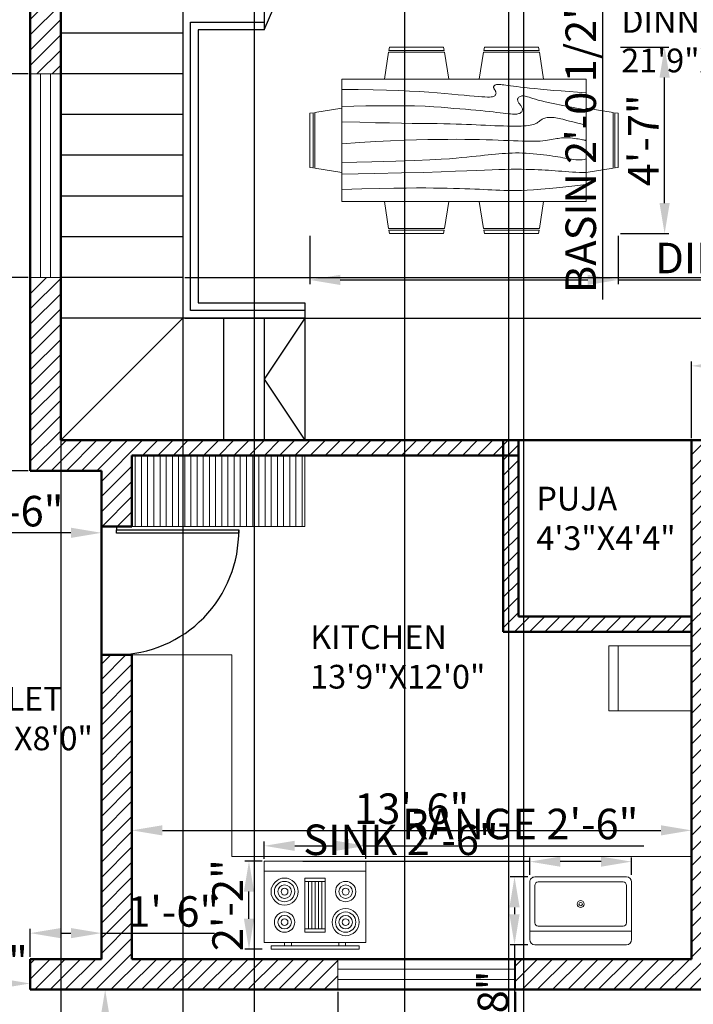
# Model space of a CAD drawing. Units: inches. Extents: x 53662 to 54269, y 37303 to 38048.
# Tile 3 of 6: x 53780 to 53979, y 37459 to 37749. Entities that reach past the tile are written whole.
import ezdxf

# ---------------------------------------------------------------- set-up
doc = ezdxf.new("R2010")
doc.units = ezdxf.units.IN
for name, color, linetype, lineweight in [('A-ANNO-DIMS', 2, 'Continuous', 18), ('A-AREA-IDEN', 7, 'Continuous', 25), ('A-CASE-PATT', 8, 'Continuous', 13), ('A-DOOR', 3, 'Continuous', 25), ('A-EQPM', 9, 'Continuous', 18), ('A-FLOR-CASE', 8, 'Continuous', 18), ('A-FLOR-FIXT', 9, 'Continuous', 18), ('A-FLOR-STRS', 7, 'Continuous', 25), ('A-FURN', 8, 'Continuous', 18), ('A-GLAZ', 4, 'Continuous', 18), ('A-WALL', 7, 'Continuous', 50)]:
    doc.layers.add(name, color=color, linetype=linetype, lineweight=lineweight)
doc.layers.add('A-WALL-PATT', color=244, linetype='Continuous', lineweight=13, true_color=0x991b1e)
doc.styles.get("Standard").update_dxf_attribs({"font": 'arial.ttf'})
doc.dimstyles.new('ISO-25', dxfattribs={"dimtxt": 9, "dimasz": 9, "dimexe": 1.25, "dimexo": 0.625, "dimtad": 1, "dimdec": 1, "dimrnd": 9, "dimlunit": 3, "dimtxsty": 'Standard', "dimcen": 2.5, "dimadec": 0, "dimazin": 0, "dimtfac": 1, "dimtdec": 1, "dimtmove": 0, "dimatfit": 3, "dimfxl": 1, "dimarcsym": 0})

# ---------------------------------------------------------------- blocks, each defined once
blk = doc.blocks.new('Dining Set - 36 x 72 in.')
for p, q in [((-22, 27.5), (-22.1562, 26.50042)), ((-5.8416, 26.5), (-22.1534, 26.5)), ((-22, 27.5), (-6, 27.5)), ((-5.8437, 26.49966), (-6, 27.5)), ((6, 27.5), (5.8438, 26.50042)), ((22.1584, 26.5), (5.8466, 26.5)), ((6, 27.5), (22, 27.5)), ((22.1563, 26.49966), (22, 27.5)), ((-22.2343, 26.00059), (-23.4847, 17.99762)), ((-22.2304, 26), (-5.7608, 26)), ((-4.5152, 17.99762), (-5.7655, 25.99926)), ((5.7657, 26.00059), (4.5153, 17.99762)), ((5.7696, 26), (22.2392, 26)), ((23.4848, 17.99762), (22.2345, 25.99926)), ((36, 18), (-36, 18)), ((-36, 18), (-36, -18)), ((36, -18), (36, 18)), ((-44.0006, 8.23428), (-35.9976, 9.48474)), ((44.0006, 8.23428), (35.9976, 9.48474)), ((-45.5, 8), (-44.5004, 8.15617)), ((-45.5, 8), (-45.5, -8)), ((-44.5, -8.15843), (-44.5, 8.15338)), ((-44, 8.23041), (-44, -8.23915)), ((44, 8.23041), (44, -8.23915)), ((44.5, -8.15843), (44.5, 8.15338)), ((45.5, 8), (44.5005, 8.15617)), ((45.5, 8), (45.5, -8)), ((-44.4997, -8.15631), (-45.5, -8)), ((-35.9976, -9.48476), (-43.9993, -8.2345)), ((35.9976, -9.48476), (43.9993, -8.2345)), ((44.4997, -8.15631), (45.5, -8)), ((-36, -18), (36, -18)), ((-22.2343, -26.0006), (-23.4847, -17.99762)), ((-4.5152, -17.99762), (-5.7655, -25.99928)), ((5.7657, -26.0006), (4.5153, -17.99762)), ((23.4848, -17.99762), (22.2345, -25.99928)), ((-22.2304, -26), (-5.7608, -26)), ((5.7696, -26), (22.2392, -26)), ((-22, -27.5), (-22.1562, -26.50044)), ((-5.8416, -26.5), (-22.1534, -26.5)), ((-22, -27.5), (-6, -27.5)), ((-5.8437, -26.49967), (-6, -27.5)), ((6, -27.5), (5.8438, -26.50044)), ((22.1584, -26.5), (5.8466, -26.5)), ((6, -27.5), (22, -27.5)), ((22.1563, -26.49967), (22, -27.5))]:
    blk.add_line(p, q)
for points in [[(-36, 15), (-31.1772, 14.97754), (-26.8079, 14.91406), (-22.8538, 14.81543), (-19.276, 14.6875), (-16.0362, 14.53613), (-13.0957, 14.36718), (-10.4159, 14.18652), (-7.9583, 14), (-5.6904, 13.81315), (-3.6035, 13.63021), (-1.6954, 13.45508), (0.0365, 13.29166), (1.5945, 13.14388), (2.9811, 13.01562), (4.1988, 12.9108), (5.25, 12.83333), (6.1393, 12.78613), (6.8802, 12.76823), (7.4883, 12.77767), (7.9792, 12.8125), (8.3685, 12.87077), (8.6719, 12.95052), (8.9049, 13.0498), (9.0833, 13.16666), (9.2205, 13.29899), (9.3216, 13.44401), (9.3895, 13.59879), (9.4271, 13.76041), (9.4373, 13.92594), (9.4232, 14.09245), (9.3875, 14.257), (9.3333, 14.41666), (9.2638, 14.56917), (9.1836, 14.71484), (9.0975, 14.85465), (9.0104, 14.98958), (8.9272, 15.1206), (8.8529, 15.2487), (8.7922, 15.37483), (8.75, 15.5), (8.7305, 15.62467), (8.7344, 15.74739), (8.7617, 15.86621), (8.8125, 15.97916), (8.8867, 16.08431), (8.9844, 16.17968), (9.1055, 16.26334), (9.25, 16.33333), (9.4189, 16.38802), (9.6172, 16.42708), (9.8506, 16.45052), (10.125, 16.45833), (10.4463, 16.45052), (10.8203, 16.42708), (11.2529, 16.38802), (11.75, 16.33333), (12.3184, 16.26318), (12.9694, 16.17838), (13.7151, 16.07991), (14.5677, 15.96875), (15.5395, 15.84586), (16.6426, 15.71224), (17.8893, 15.56884), (19.2917, 15.41666), (20.859, 15.25667), (22.5879, 15.08984), (24.4721, 14.91715), (26.5052, 14.73958), (28.6809, 14.5581), (30.9929, 14.3737), (33.4347, 14.18733), (36, 14)], [(-36, 10), (-28.9766, 10.14274), (-23.1725, 10.20442), (-18.4241, 10.19775), (-14.5677, 10.13541), (-11.4399, 10.03011), (-8.877, 9.89453), (-6.7154, 9.74137), (-4.7917, 9.58333), (-2.9698, 9.43082), (-1.2246, 9.28515), (0.4415, 9.14534), (2.026, 9.01041), (3.5266, 8.87939), (4.9408, 8.7513), (6.266, 8.62516), (7.5, 8.5), (8.6411, 8.37549), (9.6914, 8.2539), (10.6538, 8.13818), (11.5312, 8.03125), (12.3267, 7.93603), (13.043, 7.85547), (13.6831, 7.79248), (14.25, 7.75), (14.7471, 7.7303), (15.1797, 7.73307), (15.5537, 7.75732), (15.875, 7.80208), (16.1494, 7.86637), (16.3828, 7.94922), (16.5811, 8.04964), (16.75, 8.16666), (16.8944, 8.29915), (17.0143, 8.44531), (17.1089, 8.60319), (17.1771, 8.77083), (17.218, 8.94629), (17.2305, 9.1276), (17.2137, 9.31282), (17.1667, 9.5), (17.0895, 9.6875), (16.987, 9.875), (16.8649, 10.0625), (16.7292, 10.25), (16.5856, 10.4375), (16.4401, 10.625), (16.2985, 10.8125), (16.1667, 11), (16.05, 11.18733), (15.9518, 11.3737), (15.8752, 11.5581), (15.8229, 11.73958), (15.798, 11.91715), (15.8034, 12.08984), (15.842, 12.25667), (15.9167, 12.41666), (16.0295, 12.56836), (16.1784, 12.70833), (16.3605, 12.83268), (16.5729, 12.9375), (16.8127, 13.01888), (17.0768, 13.07291), (17.3625, 13.0957), (17.6667, 13.08333), (17.9894, 13.03312), (18.3418, 12.94726), (18.7382, 12.82918), (19.1927, 12.68229), (19.7195, 12.51001), (20.3327, 12.31575), (21.0465, 12.10294), (21.875, 11.875), (22.8357, 11.63354), (23.959, 11.37304), (25.2786, 11.08618), (26.8282, 10.76562), (28.6414, 10.40405), (30.752, 9.99414), (33.1936, 9.52856), (36, 9)], [(-36, 5.5), (-30.7157, 5.3348), (-26.069, 5.20963), (-21.9946, 5.11767), (-18.4271, 5.05208), (-15.3009, 5.00602), (-12.5508, 4.97265), (-10.1112, 4.94515), (-7.9167, 4.91666), (-5.909, 4.88167), (-4.0586, 4.83984), (-2.3429, 4.79215), (-0.7396, 4.73958), (0.7739, 4.6831), (2.22, 4.6237), (3.6213, 4.56233), (5, 4.5), (6.373, 4.43782), (7.7344, 4.3776), (9.0723, 4.32129), (10.375, 4.27083), (11.6309, 4.22819), (12.8281, 4.19531), (13.9551, 4.17415), (15, 4.16666), (15.954, 4.17448), (16.819, 4.19791), (17.6001, 4.23698), (18.3021, 4.29166), (18.9299, 4.36198), (19.4883, 4.44791), (19.9823, 4.54948), (20.4167, 4.66666), (20.7969, 4.79899), (21.1302, 4.94401), (21.4245, 5.09879), (21.6875, 5.26041), (21.9271, 5.42594), (22.1511, 5.59245), (22.3672, 5.757), (22.5834, 5.91666), (22.8065, 6.06868), (23.0404, 6.21093), (23.2879, 6.34147), (23.5521, 6.45833), (23.8358, 6.55957), (24.142, 6.64323), (24.4735, 6.70735), (24.8334, 6.75), (25.2235, 6.76969), (25.642, 6.76692), (26.0858, 6.74267), (26.5521, 6.69791), (27.0379, 6.63362), (27.5404, 6.55078), (28.0565, 6.45036), (28.5834, 6.33333), (29.1242, 6.19987), (29.7071, 6.04687), (30.3661, 5.87044), (31.1354, 5.66666), (32.0493, 5.43164), (33.142, 5.16146), (34.4475, 4.85221), (36, 4.5)], [(-36, -1), (-30.7915, -0.6591), (-26.0195, -0.38216), (-21.6519, -0.16284), (-17.6563, 0.00521), (-14.0005, 0.12833), (-10.6523, 0.21289), (-7.5796, 0.26522), (-4.75, 0.29166), (-2.134, 0.29793), (0.2878, 0.28711), (2.5317, 0.26163), (4.6146, 0.22396), (6.5529, 0.17651), (8.3633, 0.12174), (10.0623, 0.06209), (11.6667, 0), (13.1899, -0.06201), (14.6341, -0.1211), (15.9982, -0.17432), (17.2813, -0.21875), (18.4823, -0.25147), (19.6003, -0.26953), (20.6343, -0.27002), (21.5834, -0.25), (22.4481, -0.20768), (23.2357, -0.14584), (23.9549, -0.06836), (24.6146, 0.02083), (25.2235, 0.11784), (25.7904, 0.21875), (26.3241, 0.31966), (26.8334, 0.41666), (27.3265, 0.50618), (27.8099, 0.58593), (28.2894, 0.65397), (28.7709, 0.70833), (29.2601, 0.74707), (29.763, 0.76823), (30.2855, 0.76985), (30.8334, 0.75), (31.4088, 0.70784), (31.9994, 0.64713), (32.589, 0.57275), (33.1615, 0.48958), (33.7008, 0.4025), (34.1908, 0.3164), (34.6153, 0.23616), (34.9584, 0.16666), (35.2099, 0.11165), (35.3848, 0.07031), (35.504, 0.04069), (35.5886, 0.02083), (35.6594, 0.00879), (35.7377, 0.0026), (35.8442, 0.00032), (36, 0)], [(-36, -6.5), (-27.1843, -6.31267), (-20.084, -6.1263), (-14.469, -5.9419), (-10.1094, -5.76042), (-6.7752, -5.58285), (-4.2363, -5.41016), (-2.2629, -5.24333), (-0.625, -5.08334), (0.8708, -4.93099), (2.2715, -4.78646), (3.5872, -4.64974), (4.8281, -4.52084), (6.0046, -4.39974), (7.127, -4.28646), (8.2053, -4.18099), (9.25, -4.08334), (10.2705, -3.99382), (11.2734, -3.91407), (12.2647, -3.84603), (13.25, -3.79167), (14.2354, -3.75293), (15.2266, -3.73177), (16.2295, -3.73015), (17.25, -3.75), (18.2912, -3.79248), (19.3451, -3.85547), (20.4009, -3.93604), (21.4479, -4.03125), (22.4754, -4.13819), (23.4727, -4.25391), (24.4289, -4.37549), (25.3334, -4.5), (26.1785, -4.62492), (26.9694, -4.74935), (27.7145, -4.87281), (28.4219, -4.99479), (29.1, -5.11483), (29.7572, -5.23242), (30.4016, -5.34709), (31.0417, -5.45834), (31.6837, -5.56437), (32.3262, -5.65821), (32.9658, -5.73153), (33.599, -5.77604), (34.2224, -5.78345), (34.8327, -5.74545), (35.4264, -5.65373), (36, -5.5)], [(-36, -10), (-26.4022, -9.81299), (-18.4675, -9.62891), (-11.9839, -9.45069), (-6.7396, -9.28125), (-2.5226, -9.12354), (0.8789, -8.98047), (3.6769, -8.85498), (6.0833, -8.75), (8.2767, -8.66765), (10.3021, -8.60677), (12.1712, -8.56543), (13.8958, -8.54167), (15.4876, -8.53353), (16.9583, -8.53907), (18.3197, -8.55632), (19.5834, -8.58334), (20.7616, -8.61841), (21.8685, -8.66081), (22.9188, -8.71004), (23.9271, -8.76563), (24.9081, -8.82707), (25.8763, -8.89388), (26.8465, -8.96558), (27.8334, -9.04167), (28.8474, -9.12118), (29.8828, -9.20117), (30.93, -9.27824), (31.9792, -9.34896), (33.0205, -9.40991), (34.0443, -9.45768), (35.0407, -9.48885), (36, -9.5)], [(-36, -14.5), (-30.0881, -14.33513), (-25.0332, -14.21224), (-20.7312, -14.12647), (-17.0781, -14.07292), (-13.97, -14.04671), (-11.3027, -14.04297), (-8.9724, -14.05681), (-6.875, -14.08334), (-4.9224, -14.11833), (-3.0905, -14.16016), (-1.3709, -14.20785), (0.2448, -14.26042), (1.7647, -14.3169), (3.1973, -14.3763), (4.5507, -14.43767), (5.8333, -14.5), (7.0554, -14.5621), (8.235, -14.62175), (9.3922, -14.67652), (10.5469, -14.72396), (11.7192, -14.76164), (12.929, -14.78711), (14.1965, -14.79794), (15.5417, -14.79167), (16.9933, -14.76424), (18.6152, -14.70508), (20.4804, -14.60197), (22.6615, -14.44271), (25.2312, -14.21509), (28.2624, -13.9069), (31.8277, -13.50594), (36, -13)]]:
    blk.add_lwpolyline(points)
blk = doc.blocks.new('Sink-single - 30 in top')
blk.add_line((-15, -3.999996), (15, -3.999996))
for points in [[(-13.5, 0), (13.5, 0)], [(-15, -18.499996), (-15, -1.5)], [(15, -1.5), (15, -18.499996)], [(-12.5, -5.499996), (12.5, -5.499996)], [(-13.5, -17.499996), (-13.5, -6.499996)], [(13.5, -6.499996), (13.5, -17.499996)], [(13.5, -19.999996), (-13.5, -19.999996)], [(12.5, -18.499996), (-12.5, -18.499996)]]:
    blk.add_lwpolyline(points)
for radius in [1, 0.5]:
    blk.add_circle((0, -11.999996), radius)
for centre, radius, start, end in [((-13.5, -1.5), 1.5, 90, 180), ((13.5, -1.5), 1.5, 0, 90), ((-12.5, -6.499996), 1, 90, 180), ((12.5, -6.499996), 1, 0, 90), ((-13.5, -18.499996), 1.5, 180, 270), ((-12.5, -17.499996), 1, 180, 270), ((12.5, -17.499996), 1, 270, 0), ((13.5, -18.499996), 1.5, 270, 0)]:
    blk.add_arc(centre, radius, start, end)
blk = doc.blocks.new('Range-Oven - 30 in top')
for p, q in [((0, -3), (30, -3)), ((12, -6), (18, -6)), ((13, -20), (13, -6)), ((14, -6), (14, -20)), ((15, -20), (15, -6)), ((16, -6), (16, -20)), ((17, -20), (17, -6)), ((18, -20), (12, -20)), ((6, -24), (6, -25)), ((8, -25), (8, -24)), ((22, -25), (22, -24)), ((24, -24), (24, -25))]:
    blk.add_line(p, q)
for points in [[(0, -24), (0, 0), (30, 0), (30, -24)], [(12, -21), (12, -5), (18, -5), (18, -21)], [(2, -26), (2, -25), (28, -25), (28, -26)]]:
    blk.add_lwpolyline(points, close=True)
for centre, radius in [((6, -9), 4), ((6, -9), 3), ((6, -9), 2), ((6, -9), 1), ((24, -9), 3), ((24, -9), 2), ((24, -9), 1), ((24, -18), 4), ((6, -18), 3), ((6, -18), 2), ((6, -18), 1), ((24, -18), 3), ((24, -18), 2), ((24, -18), 1)]:
    blk.add_circle(centre, radius)
blk = doc.blocks.new('*D15')
at = {"layer": 'A-ANNO-DIMS', "color": 0, "lineweight": -2, "transparency": 16777216}
for p, q in [((53754.61, 37615.24), (53754.61, 37596.31)), ((53804.11, 37615.24), (53804.11, 37596.31)), ((53795.11, 37597.56), (53763.61, 37597.56))]:
    blk.add_line(p, q, dxfattribs=at)
at = {"layer": 'A-ANNO-DIMS', "color": 0, "transparency": 16777216}
for points in [[(53763.61, 37599.06), (53763.61, 37596.06), (53754.61, 37597.56)], [(53795.11, 37599.06), (53795.11, 37596.06), (53804.11, 37597.56)]]:
    blk.add_solid(points, dxfattribs=at)
at = {"layer": 'Defpoints', "color": 0, "transparency": 16777216}
for p in [(53754.61, 37615.86), (53804.11, 37615.86), (53754.61, 37597.56)]:
    blk.add_point(p, dxfattribs=at)
at = {"layer": 'A-ANNO-DIMS', "color": 0, "transparency": 16777216, "insert": (53779.36, 37602.78), "char_height": 9, "attachment_point": 5}
blk.add_mtext('4\'-6"', dxfattribs=at)
blk = doc.blocks.new('*D16')
at = {"layer": 'A-ANNO-DIMS', "color": 0, "lineweight": -2, "transparency": 16777216}
for p, q in [((53783.11, 37472.49), (53783.11, 37480.77)), ((53804.11, 37472.49), (53804.11, 37480.77)), ((53792.11, 37479.52), (53795.11, 37479.52)), ((53804.11, 37479.52), (53837.44, 37479.52))]:
    blk.add_line(p, q, dxfattribs=at)
at = {"layer": 'A-ANNO-DIMS', "color": 0, "transparency": 16777216}
for points in [[(53792.11, 37481.02), (53792.11, 37478.02), (53783.11, 37479.52)], [(53795.11, 37481.02), (53795.11, 37478.02), (53804.11, 37479.52)]]:
    blk.add_solid(points, dxfattribs=at)
at = {"layer": 'Defpoints', "color": 0, "transparency": 16777216}
for p in [(53804.11, 37479.52), (53783.11, 37471.86), (53804.11, 37471.86)]:
    blk.add_point(p, dxfattribs=at)
at = {"layer": 'A-ANNO-DIMS', "color": 0, "transparency": 16777216, "insert": (53825.28, 37484.74), "char_height": 9, "attachment_point": 5}
blk.add_mtext('1\'-6"', dxfattribs=at)
blk = doc.blocks.new('*D17')
at = {"layer": 'A-ANNO-DIMS', "color": 0, "lineweight": -2, "transparency": 16777216}
for p, q in [((53754.61, 37463.49), (53754.61, 37465.93)), ((53783.11, 37463.49), (53783.11, 37465.93)), ((53774.11, 37464.68), (53763.61, 37464.68))]:
    blk.add_line(p, q, dxfattribs=at)
at = {"layer": 'A-ANNO-DIMS', "color": 0, "transparency": 16777216}
for points in [[(53763.61, 37466.18), (53763.61, 37463.18), (53754.61, 37464.68)], [(53774.11, 37466.18), (53774.11, 37463.18), (53783.11, 37464.68)]]:
    blk.add_solid(points, dxfattribs=at)
at = {"layer": 'Defpoints', "color": 0, "transparency": 16777216}
for p in [(53754.61, 37464.68), (53754.61, 37462.86), (53783.11, 37462.86)]:
    blk.add_point(p, dxfattribs=at)
at = {"layer": 'A-ANNO-DIMS', "color": 0, "transparency": 16777216, "insert": (53768.86, 37469.9), "char_height": 9, "attachment_point": 5}
blk.add_mtext('2\'-3"', dxfattribs=at)
blk = doc.blocks.new('*D18')
at = {"layer": 'A-ANNO-DIMS', "color": 0, "lineweight": -2, "transparency": 16777216}
for p, q in [((53783.74, 37462.86), (53806.47, 37462.86)), ((53805.22, 37453.86), (53805.22, 37432.36)), ((53783.74, 37423.36), (53806.47, 37423.36))]:
    blk.add_line(p, q, dxfattribs=at)
at = {"layer": 'A-ANNO-DIMS', "color": 0, "transparency": 16777216}
for points in [[(53803.72, 37453.86), (53806.72, 37453.86), (53805.22, 37462.86)], [(53803.72, 37432.36), (53806.72, 37432.36), (53805.22, 37423.36)]]:
    blk.add_solid(points, dxfattribs=at)
at = {"layer": 'Defpoints', "color": 0, "transparency": 16777216}
for p in [(53783.11, 37462.86), (53783.11, 37423.36), (53805.22, 37423.36)]:
    blk.add_point(p, dxfattribs=at)
at = {"layer": 'A-ANNO-DIMS', "color": 0, "transparency": 16777216, "insert": (53799.99, 37443.11), "char_height": 9, "attachment_point": 5, "rotation": 90}
blk.add_mtext("3'", dxfattribs=at)
blk = doc.blocks.new('*D22')
at = {"layer": 'A-ANNO-DIMS', "color": 0, "lineweight": -2, "transparency": 16777216}
for p, q in [((53813.11, 37472.49), (53813.11, 37511.07)), ((53822.11, 37509.82), (53969.11, 37509.82)), ((53978.11, 37472.49), (53978.11, 37511.07))]:
    blk.add_line(p, q, dxfattribs=at)
at = {"layer": 'A-ANNO-DIMS', "color": 0, "transparency": 16777216}
for points in [[(53822.11, 37511.32), (53822.11, 37508.32), (53813.11, 37509.82)], [(53969.11, 37511.32), (53969.11, 37508.32), (53978.11, 37509.82)]]:
    blk.add_solid(points, dxfattribs=at)
at = {"layer": 'Defpoints', "color": 0, "transparency": 16777216}
for p in [(53978.11, 37509.82), (53813.11, 37471.86), (53978.11, 37471.86)]:
    blk.add_point(p, dxfattribs=at)
at = {"layer": 'A-ANNO-DIMS', "color": 0, "transparency": 16777216, "insert": (53895.61, 37515.04), "char_height": 9, "attachment_point": 5}
blk.add_mtext('13\'-6"', dxfattribs=at)
blk = doc.blocks.new('*D23')
at = {"layer": 'A-ANNO-DIMS', "color": 0, "lineweight": -2, "transparency": 16777216}
for p, q in [((53978.11, 37625.49), (53978.11, 37648.03)), ((53987.11, 37646.78), (54070.03, 37646.78)), ((54079.03, 37625.49), (54079.03, 37648.03))]:
    blk.add_line(p, q, dxfattribs=at)
at = {"layer": 'A-ANNO-DIMS', "color": 0, "transparency": 16777216}
for points in [[(53987.11, 37648.28), (53987.11, 37645.28), (53978.11, 37646.78)], [(54070.03, 37648.28), (54070.03, 37645.28), (54079.03, 37646.78)]]:
    blk.add_solid(points, dxfattribs=at)
at = {"layer": 'Defpoints', "color": 0, "transparency": 16777216}
for p in [(54079.03, 37646.78), (53978.11, 37624.86), (54079.03, 37624.86)]:
    blk.add_point(p, dxfattribs=at)
at = {"layer": 'A-ANNO-DIMS', "color": 0, "transparency": 16777216, "insert": (54028.57, 37652), "char_height": 9, "attachment_point": 5}
blk.add_mtext('8\'-3"', dxfattribs=at)
blk = doc.blocks.new('DOOR-LEAF-36IN')
for p, q in [((1, 36), (0, 36)), ((0, 36), (0, 0)), ((1, 0), (1, 36)), ((0, 0), (1, 0)), ((2, 0), (1, 0))]:
    blk.add_line(p, q)
blk = doc.blocks.new('*D34')
at = {"layer": 'A-ANNO-DIMS', "color": 0, "lineweight": -2, "transparency": 16777216}
for p, q in [((53865.53, 37685.16), (53865.53, 37670.88)), ((53956.53, 37685.16), (53956.53, 37670.88)), ((53874.53, 37672.13), (53947.53, 37672.13)), ((53956.53, 37672.13), (54065.7, 37672.13))]:
    blk.add_line(p, q, dxfattribs=at)
at = {"layer": 'A-ANNO-DIMS', "color": 0, "transparency": 16777216}
for points in [[(53874.53, 37673.63), (53874.53, 37670.63), (53865.53, 37672.13)], [(53947.53, 37673.63), (53947.53, 37670.63), (53956.53, 37672.13)]]:
    blk.add_solid(points, dxfattribs=at)
at = {"layer": 'Defpoints', "color": 0, "transparency": 16777216}
for p in [(53865.53, 37685.78), (53956.53, 37685.78), (53956.53, 37672.13)]:
    blk.add_point(p, dxfattribs=at)
at = {"layer": 'A-ANNO-DIMS', "color": 0, "transparency": 16777216, "insert": (54015.61, 37677.41), "char_height": 9, "attachment_point": 5}
blk.add_mtext('DINING SET 7\'-7"', dxfattribs=at)
blk = doc.blocks.new('*D35')
at = {"layer": 'A-ANNO-DIMS', "color": 0, "lineweight": -2, "transparency": 16777216}
for p, q in [((53957.15, 37740.78), (53971.43, 37740.78)), ((53970.18, 37694.78), (53970.18, 37731.78)), ((53957.15, 37685.78), (53971.43, 37685.78))]:
    blk.add_line(p, q, dxfattribs=at)
at = {"layer": 'A-ANNO-DIMS', "color": 0, "transparency": 16777216}
for points in [[(53968.68, 37731.78), (53971.68, 37731.78), (53970.18, 37740.78)], [(53968.68, 37694.78), (53971.68, 37694.78), (53970.18, 37685.78)]]:
    blk.add_solid(points, dxfattribs=at)
at = {"layer": 'Defpoints', "color": 0, "transparency": 16777216}
for p in [(53956.53, 37740.78), (53970.18, 37740.78), (53956.53, 37685.78)]:
    blk.add_point(p, dxfattribs=at)
at = {"layer": 'A-ANNO-DIMS', "color": 0, "transparency": 16777216, "insert": (53965.05, 37713.28), "char_height": 9, "attachment_point": 5, "rotation": 90}
blk.add_mtext('4\'-7"', dxfattribs=at)
blk = doc.blocks.new('*D38')
at = {"layer": 'A-ANNO-DIMS', "color": 0, "lineweight": -2, "transparency": 16777216}
for p, q in [((53948.84, 37817.85), (53953.14, 37817.85)), ((53951.89, 37808.85), (53951.89, 37802.3)), ((53948.84, 37793.3), (53953.14, 37793.3)), ((53951.89, 37793.3), (53951.89, 37666.39))]:
    blk.add_line(p, q, dxfattribs=at)
at = {"layer": 'A-ANNO-DIMS', "color": 0, "transparency": 16777216}
for points in [[(53950.39, 37808.85), (53953.39, 37808.85), (53951.89, 37817.85)], [(53950.39, 37802.3), (53953.39, 37802.3), (53951.89, 37793.3)]]:
    blk.add_solid(points, dxfattribs=at)
at = {"layer": 'Defpoints', "color": 0, "transparency": 16777216}
for p in [(53948.21, 37817.85), (53948.21, 37793.3), (53951.89, 37793.3)]:
    blk.add_point(p, dxfattribs=at)
at = {"layer": 'A-ANNO-DIMS', "color": 0, "transparency": 16777216, "insert": (53946.62, 37725.34), "char_height": 9, "attachment_point": 5, "rotation": 90}
blk.add_mtext('BASIN 2\'-0 1/2" TYP.', dxfattribs=at)
blk = doc.blocks.new('*D44')
at = {"layer": 'A-ANNO-DIMS', "color": 0, "lineweight": -2, "transparency": 16777216}
for p, q in [((53930.43, 37500.6), (53863.46, 37500.6)), ((53930.43, 37496.73), (53930.43, 37501.85)), ((53951.43, 37500.6), (53939.43, 37500.6)), ((53960.43, 37496.73), (53960.43, 37501.85))]:
    blk.add_line(p, q, dxfattribs=at)
at = {"layer": 'A-ANNO-DIMS', "color": 0, "transparency": 16777216}
for points in [[(53939.43, 37502.1), (53939.43, 37499.1), (53930.43, 37500.6)], [(53951.43, 37502.1), (53951.43, 37499.1), (53960.43, 37500.6)]]:
    blk.add_solid(points, dxfattribs=at)
at = {"layer": 'Defpoints', "color": 0, "transparency": 16777216}
for p in [(53930.43, 37500.6), (53930.43, 37496.1), (53960.43, 37496.1)]:
    blk.add_point(p, dxfattribs=at)
at = {"layer": 'A-ANNO-DIMS', "color": 0, "transparency": 16777216, "insert": (53892.45, 37505.88), "char_height": 9, "attachment_point": 5}
blk.add_mtext('SINK 2\'-6"', dxfattribs=at)
blk = doc.blocks.new('*D45')
at = {"layer": 'A-ANNO-DIMS', "color": 0, "lineweight": -2, "transparency": 16777216}
for p, q in [((53929.81, 37496.1), (53924.68, 37496.1)), ((53925.93, 37487.1), (53925.93, 37485.1)), ((53929.81, 37476.1), (53924.68, 37476.1)), ((53925.93, 37476.1), (53925.93, 37442.77))]:
    blk.add_line(p, q, dxfattribs=at)
at = {"layer": 'A-ANNO-DIMS', "color": 0, "transparency": 16777216}
for points in [[(53924.43, 37487.1), (53927.43, 37487.1), (53925.93, 37496.1)], [(53924.43, 37485.1), (53927.43, 37485.1), (53925.93, 37476.1)]]:
    blk.add_solid(points, dxfattribs=at)
at = {"layer": 'Defpoints', "color": 0, "transparency": 16777216}
for p in [(53930.43, 37496.1), (53925.93, 37476.1), (53930.43, 37476.1)]:
    blk.add_point(p, dxfattribs=at)
at = {"layer": 'A-ANNO-DIMS', "color": 0, "transparency": 16777216, "insert": (53920.71, 37454.94), "char_height": 9, "attachment_point": 5, "rotation": 90}
blk.add_mtext('1\'-8"', dxfattribs=at)
blk = doc.blocks.new('*D46')
at = {"layer": 'A-ANNO-DIMS', "color": 0, "lineweight": -2, "transparency": 16777216}
for p, q in [((53852.13, 37501.39), (53852.13, 37506.51)), ((53882.13, 37501.39), (53882.13, 37506.51)), ((53861.13, 37505.26), (53873.13, 37505.26)), ((53882.13, 37505.26), (53964.05, 37505.26))]:
    blk.add_line(p, q, dxfattribs=at)
at = {"layer": 'A-ANNO-DIMS', "color": 0, "transparency": 16777216}
for points in [[(53861.13, 37506.76), (53861.13, 37503.76), (53852.13, 37505.26)], [(53873.13, 37506.76), (53873.13, 37503.76), (53882.13, 37505.26)]]:
    blk.add_solid(points, dxfattribs=at)
at = {"layer": 'Defpoints', "color": 0, "transparency": 16777216}
for p in [(53882.13, 37505.26), (53852.13, 37500.76), (53882.13, 37500.76)]:
    blk.add_point(p, dxfattribs=at)
at = {"layer": 'A-ANNO-DIMS', "color": 0, "transparency": 16777216, "insert": (53927.59, 37510.54), "char_height": 9, "attachment_point": 5}
blk.add_mtext('RANGE 2\'-6"', dxfattribs=at)
blk = doc.blocks.new('*D47')
at = {"layer": 'A-ANNO-DIMS', "color": 0, "lineweight": -2, "transparency": 16777216}
for p, q in [((53851.51, 37500.76), (53846.38, 37500.76)), ((53847.63, 37483.76), (53847.63, 37491.76)), ((53851.51, 37474.76), (53846.38, 37474.76))]:
    blk.add_line(p, q, dxfattribs=at)
at = {"layer": 'A-ANNO-DIMS', "color": 0, "transparency": 16777216}
for points in [[(53846.13, 37491.76), (53849.13, 37491.76), (53847.63, 37500.76)], [(53846.13, 37483.76), (53849.13, 37483.76), (53847.63, 37474.76)]]:
    blk.add_solid(points, dxfattribs=at)
at = {"layer": 'Defpoints', "color": 0, "transparency": 16777216}
for p in [(53847.63, 37500.76), (53852.13, 37500.76), (53852.13, 37474.76)]:
    blk.add_point(p, dxfattribs=at)
at = {"layer": 'A-ANNO-DIMS', "color": 0, "transparency": 16777216, "insert": (53842.49, 37487.76), "char_height": 9, "attachment_point": 5, "rotation": 90}
blk.add_mtext('2\'-2"', dxfattribs=at)
blk = doc.blocks.new('*D52')
at = {"layer": 'A-ANNO-DIMS', "color": 0, "lineweight": -2, "transparency": 16777216}
for p, q in [((53792.11, 37660.24), (53792.11, 37309.49)), ((53828.11, 37660.24), (53828.11, 37309.49)), ((53801.11, 37310.74), (53819.11, 37310.74))]:
    blk.add_line(p, q, dxfattribs=at)
at = {"layer": 'A-ANNO-DIMS', "color": 0, "transparency": 16777216}
for points in [[(53801.11, 37312.24), (53801.11, 37309.24), (53792.11, 37310.74)], [(53819.11, 37312.24), (53819.11, 37309.24), (53828.11, 37310.74)]]:
    blk.add_solid(points, dxfattribs=at)
at = {"layer": 'Defpoints', "color": 0, "transparency": 16777216}
for p in [(53792.11, 37660.86), (53828.11, 37660.86), (53828.11, 37310.74)]:
    blk.add_point(p, dxfattribs=at)
at = {"layer": 'A-ANNO-DIMS', "color": 0, "transparency": 16777216, "insert": (53810.11, 37315.96), "char_height": 9, "attachment_point": 5}
blk.add_mtext('3\'-0"', dxfattribs=at)
blk = doc.blocks.new('*D53')
at = {"layer": 'A-ANNO-DIMS', "color": 0, "lineweight": -2, "transparency": 16777216}
for p, q in [((54260.82, 37681.86), (54260.82, 37715.19)), ((53828.74, 37672.86), (54262.07, 37672.86)), ((54260.82, 37660.86), (54260.82, 37672.86)), ((53828.74, 37660.86), (54262.07, 37660.86)), ((54260.82, 37651.86), (54260.82, 37642.86))]:
    blk.add_line(p, q, dxfattribs=at)
at = {"layer": 'A-ANNO-DIMS', "color": 0, "transparency": 16777216}
for points in [[(54259.32, 37681.86), (54262.32, 37681.86), (54260.82, 37672.86)], [(54259.32, 37651.86), (54262.32, 37651.86), (54260.82, 37660.86)]]:
    blk.add_solid(points, dxfattribs=at)
at = {"layer": 'Defpoints', "color": 0, "transparency": 16777216}
for p in [(53828.11, 37672.86), (54260.82, 37672.86), (53828.11, 37660.86)]:
    blk.add_point(p, dxfattribs=at)
at = {"layer": 'A-ANNO-DIMS', "color": 0, "transparency": 16777216, "insert": (54255.6, 37703.02), "char_height": 9, "attachment_point": 5, "rotation": 90}
blk.add_mtext('1\'-0"', dxfattribs=at)
blk = doc.blocks.new('*D54')
at = {"layer": 'A-ANNO-DIMS', "color": 0, "lineweight": -2, "transparency": 16777216}
for p, q in [((53792.11, 37952.24), (53792.11, 37309.49)), ((53849.2, 37952.24), (53849.2, 37309.49)), ((53801.11, 37310.74), (53840.2, 37310.74))]:
    blk.add_line(p, q, dxfattribs=at)
at = {"layer": 'A-ANNO-DIMS', "color": 0, "transparency": 16777216}
for points in [[(53801.11, 37312.24), (53801.11, 37309.24), (53792.11, 37310.74)], [(53840.2, 37312.24), (53840.2, 37309.24), (53849.2, 37310.74)]]:
    blk.add_solid(points, dxfattribs=at)
at = {"layer": 'Defpoints', "color": 0, "transparency": 16777216}
for p in [(53792.11, 37952.86), (53849.2, 37952.86), (53849.2, 37310.74)]:
    blk.add_point(p, dxfattribs=at)
at = {"layer": 'A-ANNO-DIMS', "color": 0, "transparency": 16777216, "insert": (53820.66, 37315.96), "char_height": 9, "attachment_point": 5}
blk.add_mtext('4\'-9"', dxfattribs=at)
blk = doc.blocks.new('*D55')
at = {"layer": 'A-ANNO-DIMS', "color": 0, "lineweight": -2, "transparency": 16777216}
for p, q in [((53849.2, 37952.24), (53849.2, 37309.49)), ((53893.52, 37952.24), (53893.52, 37309.49)), ((53858.2, 37310.74), (53884.52, 37310.74)), ((53893.52, 37310.74), (53948.66, 37310.74))]:
    blk.add_line(p, q, dxfattribs=at)
at = {"layer": 'A-ANNO-DIMS', "color": 0, "transparency": 16777216}
for points in [[(53858.2, 37312.24), (53858.2, 37309.24), (53849.2, 37310.74)], [(53884.52, 37312.24), (53884.52, 37309.24), (53893.52, 37310.74)]]:
    blk.add_solid(points, dxfattribs=at)
at = {"layer": 'Defpoints', "color": 0, "transparency": 16777216}
for p in [(53849.2, 37952.86), (53893.52, 37952.86), (53893.52, 37310.74)]:
    blk.add_point(p, dxfattribs=at)
at = {"layer": 'A-ANNO-DIMS', "color": 0, "transparency": 16777216, "insert": (53925.59, 37316.02), "char_height": 9, "attachment_point": 5}
blk.add_mtext('3\'-8 1/2"', dxfattribs=at)
blk = doc.blocks.new('*D60')
at = {"layer": 'A-ANNO-DIMS', "color": 0, "lineweight": -2, "transparency": 16777216}
for p, q in [((53924.11, 37790.24), (53924.11, 37309.49)), ((53928.61, 37790.24), (53928.61, 37309.49)), ((53915.11, 37310.74), (53906.11, 37310.74)), ((53924.11, 37310.74), (53928.61, 37310.74)), ((53937.61, 37310.74), (53992.76, 37310.74))]:
    blk.add_line(p, q, dxfattribs=at)
at = {"layer": 'A-ANNO-DIMS', "color": 0, "transparency": 16777216}
for points in [[(53915.11, 37312.24), (53915.11, 37309.24), (53924.11, 37310.74)], [(53937.61, 37312.24), (53937.61, 37309.24), (53928.61, 37310.74)]]:
    blk.add_solid(points, dxfattribs=at)
at = {"layer": 'Defpoints', "color": 0, "transparency": 16777216}
for p in [(53924.11, 37790.86), (53928.61, 37790.86), (53928.61, 37310.74)]:
    blk.add_point(p, dxfattribs=at)
at = {"layer": 'A-ANNO-DIMS', "color": 0, "transparency": 16777216, "insert": (53969.69, 37316.02), "char_height": 9, "attachment_point": 5}
blk.add_mtext('0\'-4 1/2"', dxfattribs=at)
blk = doc.blocks.new('*D64')
at = {"layer": 'A-ANNO-DIMS', "color": 0, "lineweight": -2, "transparency": 16777216}
for p, q in [((53782.49, 37672.86), (53679.5, 37672.86)), ((53680.75, 37624.86), (53680.75, 37663.86)), ((53782.49, 37615.86), (53679.5, 37615.86))]:
    blk.add_line(p, q, dxfattribs=at)
at = {"layer": 'A-ANNO-DIMS', "color": 0, "transparency": 16777216}
for points in [[(53679.25, 37663.86), (53682.25, 37663.86), (53680.75, 37672.86)], [(53679.25, 37624.86), (53682.25, 37624.86), (53680.75, 37615.86)]]:
    blk.add_solid(points, dxfattribs=at)
at = {"layer": 'Defpoints', "color": 0, "transparency": 16777216}
for p in [(53680.75, 37672.86), (53783.11, 37672.86), (53783.11, 37615.86)]:
    blk.add_point(p, dxfattribs=at)
at = {"layer": 'A-ANNO-DIMS', "color": 0, "transparency": 16777216, "insert": (53675.53, 37644.36), "char_height": 9, "attachment_point": 5, "rotation": 90}
blk.add_mtext('4\'-9"', dxfattribs=at)
blk = doc.blocks.new('*D65')
at = {"layer": 'A-ANNO-DIMS', "color": 0, "lineweight": -2, "transparency": 16777216}
for p, q in [((53782.49, 37732.86), (53679.5, 37732.86)), ((53680.75, 37681.86), (53680.75, 37723.86)), ((53782.49, 37672.86), (53679.5, 37672.86))]:
    blk.add_line(p, q, dxfattribs=at)
at = {"layer": 'A-ANNO-DIMS', "color": 0, "transparency": 16777216}
for points in [[(53679.25, 37723.86), (53682.25, 37723.86), (53680.75, 37732.86)], [(53679.25, 37681.86), (53682.25, 37681.86), (53680.75, 37672.86)]]:
    blk.add_solid(points, dxfattribs=at)
at = {"layer": 'Defpoints', "color": 0, "transparency": 16777216}
for p in [(53680.75, 37732.86), (53783.11, 37732.86), (53783.11, 37672.86)]:
    blk.add_point(p, dxfattribs=at)
at = {"layer": 'A-ANNO-DIMS', "color": 0, "transparency": 16777216, "insert": (53675.53, 37702.86), "char_height": 9, "attachment_point": 5, "rotation": 90}
blk.add_mtext('5\'-0"', dxfattribs=at)
blk = doc.blocks.new('*D70')
at = {"layer": 'A-ANNO-DIMS', "color": 0, "lineweight": -2, "transparency": 16777216}
for p, q in [((53873.85, 37462.24), (53873.85, 37309.49)), ((53926.17, 37462.24), (53926.17, 37309.49)), ((53882.85, 37310.74), (53917.17, 37310.74))]:
    blk.add_line(p, q, dxfattribs=at)
at = {"layer": 'A-ANNO-DIMS', "color": 0, "transparency": 16777216}
for points in [[(53882.85, 37312.24), (53882.85, 37309.24), (53873.85, 37310.74)], [(53917.17, 37312.24), (53917.17, 37309.24), (53926.17, 37310.74)]]:
    blk.add_solid(points, dxfattribs=at)
at = {"layer": 'Defpoints', "color": 0, "transparency": 16777216}
for p in [(53873.85, 37462.86), (53926.17, 37462.86), (53926.17, 37310.74)]:
    blk.add_point(p, dxfattribs=at)
at = {"layer": 'A-ANNO-DIMS', "color": 0, "transparency": 16777216, "insert": (53900.01, 37316.02), "char_height": 9, "attachment_point": 5}
blk.add_mtext('4\'-4 1/2"', dxfattribs=at)
blk = doc.blocks.new('*D71')
at = {"layer": 'A-ANNO-DIMS', "color": 0, "lineweight": -2, "transparency": 16777216}
for p, q in [((53926.17, 37462.24), (53926.17, 37309.49)), ((53987.11, 37462.24), (53987.11, 37309.49)), ((53935.17, 37310.74), (53978.11, 37310.74))]:
    blk.add_line(p, q, dxfattribs=at)
at = {"layer": 'A-ANNO-DIMS', "color": 0, "transparency": 16777216}
for points in [[(53935.17, 37312.24), (53935.17, 37309.24), (53926.17, 37310.74)], [(53978.11, 37312.24), (53978.11, 37309.24), (53987.11, 37310.74)]]:
    blk.add_solid(points, dxfattribs=at)
at = {"layer": 'Defpoints', "color": 0, "transparency": 16777216}
for p in [(53926.17, 37462.86), (53987.11, 37462.86), (53987.11, 37310.74)]:
    blk.add_point(p, dxfattribs=at)
at = {"layer": 'A-ANNO-DIMS', "color": 0, "transparency": 16777216, "insert": (53956.64, 37315.96), "char_height": 9, "attachment_point": 5}
blk.add_mtext('5\'-1"', dxfattribs=at)

msp = doc.modelspace()

# ---------------------------------------------------------------- hatches: boundary and pattern name
at = {"layer": 'A-CASE-PATT'}
h = msp.add_hatch(dxfattribs=at)
h.set_pattern_fill('ANSI31', color=256, scale=0.5736783, angle=45, style=0)
h.paths.add_polyline_path([(53813.11, 37599.43), (53864.11, 37599.43), (53864.11, 37620.36), (53813.11, 37620.36)])
at = {"layer": 'A-WALL-PATT'}
h = msp.add_hatch(dxfattribs=at)
h.set_pattern_fill('ANSI31', color=256)
h.paths.add_polyline_path([(53792.11, 37952.86), (53849.2, 37952.86), (53849.2, 37961.86), (53783.11, 37961.86), (53783.11, 37861.42), (53792.11, 37861.42)])
h.paths.add_polyline_path([(53940.97, 37961.86), (53893.52, 37961.86), (53893.52, 37952.86), (53924.11, 37952.86), (53924.11, 37921.83), (53926.36, 37921.83, -0.026334), (53928.61, 37921.99), (53928.61, 37930.37), (53928.61, 37952.86), (53940.97, 37952.86)])
h.paths.add_polyline_path([(53792.11, 37786.36), (53882.05, 37786.36), (53882.05, 37788.61, -0.017862), (53881.82, 37790.86), (53792.11, 37790.86), (53792.11, 37806.76), (53783.11, 37806.76), (53783.11, 37732.86), (53792.11, 37732.86)])
h.paths.add_polyline_path([(53792.11, 37672.86), (53783.11, 37672.86), (53783.11, 37615.86), (53804.11, 37615.86), (53804.11, 37599.43), (53813.11, 37599.43), (53813.11, 37620.36), (53922.61, 37620.36), (53922.61, 37624.86), (53792.11, 37624.86)])
h.paths.add_polyline_path([(53978.11, 37572.86), (53927.11, 37572.86), (53927.11, 37620.36), (53922.61, 37620.36), (53922.61, 37568.36), (53978.11, 37568.36)])
h.paths.add_polyline_path([(53927.11, 37624.86), (53922.61, 37624.86), (53922.61, 37620.36), (53927.11, 37620.36)])
h.paths.add_polyline_path([(53987.11, 37615.86), (54079.03, 37615.86), (54079.03, 37624.86), (53978.11, 37624.86), (53978.11, 37471.86), (53926.17, 37471.86), (53926.17, 37462.86), (53987.11, 37462.86)])
h.paths.add_polyline_path([(53813.11, 37561.58), (53804.11, 37561.58), (53804.11, 37471.86), (53783.11, 37471.86), (53783.11, 37462.86), (53873.85, 37462.86), (53873.85, 37471.86), (53813.11, 37471.86)])
h.paths.add_polyline_path([(54146.11, 37687.42), (54137.11, 37687.42), (54137.11, 37624.86), (54128.99, 37624.86), (54128.99, 37615.86), (54146.11, 37615.86)])
h.paths.add_polyline_path([(54146.11, 37813.18), (54137.11, 37813.18), (54137.11, 37747.89), (54146.11, 37747.89)])
h.paths.add_polyline_path([(54146.11, 37961.86), (54107.27, 37961.86), (54107.27, 37952.86), (54137.11, 37952.86), (54137.11, 37884.55), (54146.11, 37884.55)])
h.paths.add_polyline_path([(54022.12, 37961.86), (53964.61, 37961.86), (53964.61, 37952.86), (53982.61, 37952.86), (53982.61, 37822.8), (53987.11, 37822.8), (53987.11, 37952.86), (54022.12, 37952.86)])
h.paths.add_polyline_path([(53928.61, 37899.06), (53924.11, 37899.06), (53924.11, 37790.86), (53914.92, 37790.86), (53914.92, 37786.36), (53987.11, 37786.36), (53987.11, 37797.48), (53982.61, 37797.48), (53982.61, 37790.86), (53928.61, 37790.86), (53928.61, 37801.6, -0.072813), (53928.13, 37805.9, -0.05664), (53928.61, 37809.23)])

# ---------------------------------------------------------------- linework, layer by layer
at = {"layer": 'A-DOOR'}
msp.add_arc((53808.27, 37597.93), 36.35, 270.5504, 0.7881, dxfattribs=at)
at = {"layer": 'A-FLOR-CASE'}
for p, q in [((53864.11, 37620.36), (53864.11, 37599.43)), ((53864.11, 37599.43), (53813.11, 37599.43)), ((53978.11, 37564.22), (53953.75, 37564.22)), ((53953.75, 37564.22), (53953.75, 37545.1)), ((53956.53, 37545.1), (53956.53, 37564.22)), ((53813.11, 37561.58), (53842.61, 37561.58)), ((53842.61, 37561.58), (53842.61, 37502.16)), ((53953.75, 37545.1), (53978.11, 37545.1)), ((53842.61, 37502.16), (53978.11, 37502.16))]:
    msp.add_line(p, q, dxfattribs=at)
at = {"layer": 'A-FLOR-STRS'}
for p, q in [((53828.11, 37786.36), (53828.11, 37624.86)), ((53852.11, 37786.36), (53852.11, 37745.86)), ((53852.11, 37745.86), (53860.44, 37765.15)), ((53830.36, 37663.11), (53830.36, 37748.11)), ((53830.36, 37748.11), (53852.11, 37748.11)), ((53828.11, 37744.86), (53792.11, 37744.86)), ((53852.11, 37745.86), (53832.61, 37745.86)), ((53832.61, 37745.86), (53832.61, 37665.36)), ((53828.11, 37732.86), (53792.11, 37732.86)), ((53828.11, 37720.86), (53792.11, 37720.86)), ((53828.11, 37708.86), (53792.11, 37708.86)), ((53828.11, 37696.86), (53792.11, 37696.86)), ((53828.11, 37684.86), (53792.11, 37684.86)), ((53828.11, 37672.86), (53792.11, 37672.86)), ((53864.11, 37663.11), (53830.36, 37663.11)), ((53832.61, 37665.36), (53864.11, 37665.36)), ((53864.11, 37665.36), (53864.11, 37660.86)), ((53864.11, 37660.86), (53792.11, 37660.86)), ((53828.11, 37660.86), (53792.11, 37624.86)), ((53840.11, 37660.86), (53840.11, 37624.86)), ((53852.11, 37660.86), (53852.11, 37624.86)), ((53864.11, 37660.86), (53852.11, 37642.86)), ((53864.11, 37660.86), (53864.11, 37624.86)), ((53852.11, 37642.86), (53864.11, 37624.86))]:
    msp.add_line(p, q, dxfattribs=at)
at = {"layer": 'A-GLAZ'}
for p, q in [((53792.11, 37732.86), (53783.11, 37732.86)), ((53786.11, 37732.86), (53786.11, 37672.86)), ((53789.11, 37732.86), (53789.11, 37672.86)), ((53792.11, 37672.86), (53783.11, 37672.86)), ((53873.85, 37471.86), (53873.85, 37462.86)), ((53926.17, 37471.86), (53926.17, 37462.86)), ((53926.17, 37468.86), (53873.85, 37468.86)), ((53926.17, 37465.86), (53873.85, 37465.86))]:
    msp.add_line(p, q, dxfattribs=at)
at = {"layer": 'A-WALL'}
for p, q in [((53783.11, 37961.86), (53783.11, 37615.86)), ((53792.11, 37786.36), (53792.11, 37624.86)), ((53927.11, 37624.86), (53792.11, 37624.86)), ((53922.61, 37568.36), (53922.61, 37624.86)), ((53927.11, 37624.86), (53978.11, 37624.86)), ((53927.11, 37572.86), (53927.11, 37624.86)), ((53978.11, 37471.86), (53978.11, 37624.86)), ((54079.03, 37624.86), (53978.11, 37624.86)), ((53927.11, 37620.36), (53813.11, 37620.36)), ((53813.11, 37599.43), (53813.11, 37620.36)), ((53804.11, 37615.86), (53783.11, 37615.86)), ((53804.11, 37471.86), (53804.11, 37615.86)), ((53813.11, 37599.43), (53804.11, 37599.43)), ((53927.11, 37572.86), (53978.11, 37572.86)), ((53922.61, 37568.36), (53978.11, 37568.36)), ((53813.11, 37561.58), (53804.11, 37561.58)), ((53813.11, 37471.86), (53813.11, 37561.58)), ((53783.11, 37471.86), (53783.11, 37462.86)), ((53804.11, 37471.86), (53783.11, 37471.86)), ((53978.11, 37471.86), (53813.11, 37471.86)), ((53987.11, 37462.86), (53783.11, 37462.86))]:
    msp.add_line(p, q, dxfattribs=at)

# ---------------------------------------------------------------- block references
at = {"layer": 'A-DOOR', "extrusion": (0, 0, -1), "zscale": -1, "rotation": 89.9999999999801}
msp.add_blockref('DOOR-LEAF-36IN', (-53808.61, 37597.43), dxfattribs=at)
at = {"layer": 'A-EQPM'}
msp.add_blockref('Range-Oven - 30 in top', (53852.13, 37500.76), dxfattribs=at)
at = {"layer": 'A-FLOR-FIXT', "rotation": 180}
msp.add_blockref('Sink-single - 30 in top', (53945.43, 37476.1), dxfattribs=at)
at = {"layer": 'A-FURN'}
msp.add_blockref('Dining Set - 36 x 72 in.', (53911.03, 37713.28), dxfattribs=at)

# ---------------------------------------------------------------- texts
at = {"layer": 'A-AREA-IDEN', "char_height": 7, "attachment_point": 1}
for s, width, insert in [('DINNING/DRAWING\\P21\'9"X12\'0"', 148.2626, (53957.4, 37752.01)), ('PUJA\\P4\'3"X4\'4"', 40.1945, (53932.38, 37611.14)), ('KITCHEN\\P13\'9"X12\'0"', 64.9084, (53865.69, 37570.29)), ('TOILET\\P4\'6"X8\'0"', 40.1945, (53760.56, 37552.11))]:
    msp.add_mtext_dynamic_manual_height_columns(s, width=width, gutter_width=12.5, heights=[0], dxfattribs=dict(at, insert=insert))

# ---------------------------------------------------------------- dimensions: what is measured, and where the dimension line sits
at = {"layer": 'A-ANNO-DIMS'}
for base, p1, p2, override, picture, middle in [((53849.2, 37310.74), (53792.11, 37952.86), (53849.2, 37952.86), {"dimdec": 1, "dimlfac": 1, "dimrnd": 0, "dimzin": 1, "dimdsep": 46, "dimlunit": 4, "dimfrac": 2}, '*D54', (53820.66, 37315.96)), ((53893.52, 37310.74), (53849.2, 37952.86), (53893.52, 37952.86), {"dimdec": 1, "dimlfac": 1, "dimrnd": 0, "dimzin": 1, "dimdsep": 46, "dimlunit": 4, "dimfrac": 2}, '*D55', (53925.59, 37316.02)), ((53928.61, 37310.74), (53924.11, 37790.86), (53928.61, 37790.86), {"dimdec": 1, "dimlfac": 1, "dimrnd": 0, "dimzin": 1, "dimdsep": 46, "dimlunit": 4, "dimfrac": 2}, '*D60', (53969.69, 37316.02)), ((53828.11, 37310.74), (53792.11, 37660.86), (53828.11, 37660.86), {"dimdec": 1, "dimlfac": 1, "dimrnd": 0, "dimzin": 1, "dimdsep": 46, "dimlunit": 4, "dimfrac": 2}, '*D52', (53810.11, 37315.96)), ((54079.03, 37646.78), (53978.11, 37624.86), (54079.03, 37624.86), {"dimclrd": 0, "dimclre": 0, "dimclrt": 0}, '*D23', (54028.57, 37652)), ((53754.61, 37597.56), (53804.11, 37615.86), (53754.61, 37615.86), {"dimclrd": 0, "dimclre": 0, "dimclrt": 0}, '*D15', (53779.36, 37602.78)), ((53978.11, 37509.82), (53813.11, 37471.86), (53978.11, 37471.86), {"dimclrd": 0, "dimclre": 0, "dimclrt": 0}, '*D22', (53895.61, 37515.04)), ((53804.11, 37479.52), (53783.11, 37471.86), (53804.11, 37471.86), {"dimclrd": 0, "dimclre": 0, "dimclrt": 0}, '*D16', (53825.28, 37484.74)), ((53754.61, 37464.68), (53783.11, 37462.86), (53754.61, 37462.86), {"dimclrd": 0, "dimclre": 0, "dimclrt": 0}, '*D17', (53768.86, 37469.9)), ((53926.17, 37310.74), (53873.85, 37462.86), (53926.17, 37462.86), {"dimdec": 1, "dimlfac": 1, "dimrnd": 0, "dimzin": 1, "dimdsep": 46, "dimlunit": 4, "dimfrac": 2}, '*D70', (53900.01, 37316.02)), ((53987.11, 37310.74), (53926.17, 37462.86), (53987.11, 37462.86), {"dimdec": 1, "dimlfac": 1, "dimrnd": 0, "dimzin": 1, "dimdsep": 46, "dimlunit": 4, "dimfrac": 2}, '*D71', (53956.64, 37315.96))]:
    dim = msp.add_linear_dim(base=base, p1=p1, p2=p2, dimstyle='ISO-25', override=override, dxfattribs=at)
    dim.commit()
    dim.dimension.update_dxf_attribs({"geometry": picture, "text_midpoint": middle})
for base, p1, p2, angle, text, picture, middle in [((53951.894, 37793.2972), (53948.2113, 37817.8481), (53948.2113, 37793.2972), 270, 'BASIN <> TYP.', '*D38', (53946.6155, 37725.3441)), ((53930.43, 37500.6), (53960.43, 37496.1), (53930.43, 37496.1), 180, 'SINK <>', '*D44', (53892.45, 37505.88))]:
    dim = msp.add_linear_dim(base=base, p1=p1, p2=p2, angle=angle, text=text, dimstyle='ISO-25', override={"dimdec": 1, "dimlfac": 1, "dimrnd": 0, "dimzin": 1, "dimdsep": 46, "dimlunit": 4, "dimfrac": 2}, dxfattribs=at)
    dim.commit()
    dim.dimension.update_dxf_attribs({"geometry": picture, "text_midpoint": middle})
for base, p1, p2, angle, picture, middle in [((53970.18, 37740.78), (53956.53, 37685.78), (53956.53, 37740.78), 90, '*D35', (53965.05, 37713.28)), ((53680.75, 37732.86), (53783.11, 37672.86), (53783.11, 37732.86), 90, '*D65', (53675.53, 37702.86)), ((54260.82, 37672.86), (53828.11, 37660.86), (53828.11, 37672.86), 90, '*D53', (54255.6, 37703.02)), ((53680.75, 37672.86), (53783.11, 37615.86), (53783.11, 37672.86), 90, '*D64', (53675.53, 37644.36)), ((53847.63, 37500.76), (53852.13, 37474.76), (53852.13, 37500.76), 90, '*D47', (53842.49, 37487.76)), ((53925.93, 37476.1), (53930.43, 37496.1), (53930.43, 37476.1), 270, '*D45', (53920.71, 37454.94))]:
    dim = msp.add_linear_dim(base=base, p1=p1, p2=p2, angle=angle, dimstyle='ISO-25', override={"dimdec": 1, "dimlfac": 1, "dimrnd": 0, "dimzin": 1, "dimdsep": 46, "dimlunit": 4, "dimfrac": 2}, dxfattribs=at)
    dim.commit()
    dim.dimension.update_dxf_attribs({"geometry": picture, "text_midpoint": middle})
for base, p1, p2, text, picture, middle in [((53956.53, 37672.13), (53865.53, 37685.78), (53956.53, 37685.78), 'DINING SET <>', '*D34', (54015.61, 37677.41)), ((53882.13, 37505.26), (53852.13, 37500.76), (53882.13, 37500.76), 'RANGE <>', '*D46', (53927.59, 37510.54))]:
    dim = msp.add_linear_dim(base=base, p1=p1, p2=p2, text=text, dimstyle='ISO-25', override={"dimdec": 1, "dimlfac": 1, "dimrnd": 0, "dimzin": 1, "dimdsep": 46, "dimlunit": 4, "dimfrac": 2}, dxfattribs=at)
    dim.commit()
    dim.dimension.update_dxf_attribs({"geometry": picture, "text_midpoint": middle})
dim = msp.add_aligned_dim(p1=(53783.11, 37462.86), p2=(53783.11, 37423.36), distance=22.1, dimstyle='ISO-25', override={"dimclrd": 0, "dimclre": 0, "dimclrt": 0}, dxfattribs=at)
dim.commit()
dim.dimension.update_dxf_attribs({"geometry": '*D18', "text_midpoint": (53799.99, 37443.11)})

doc.saveas('drawing.dxf')
